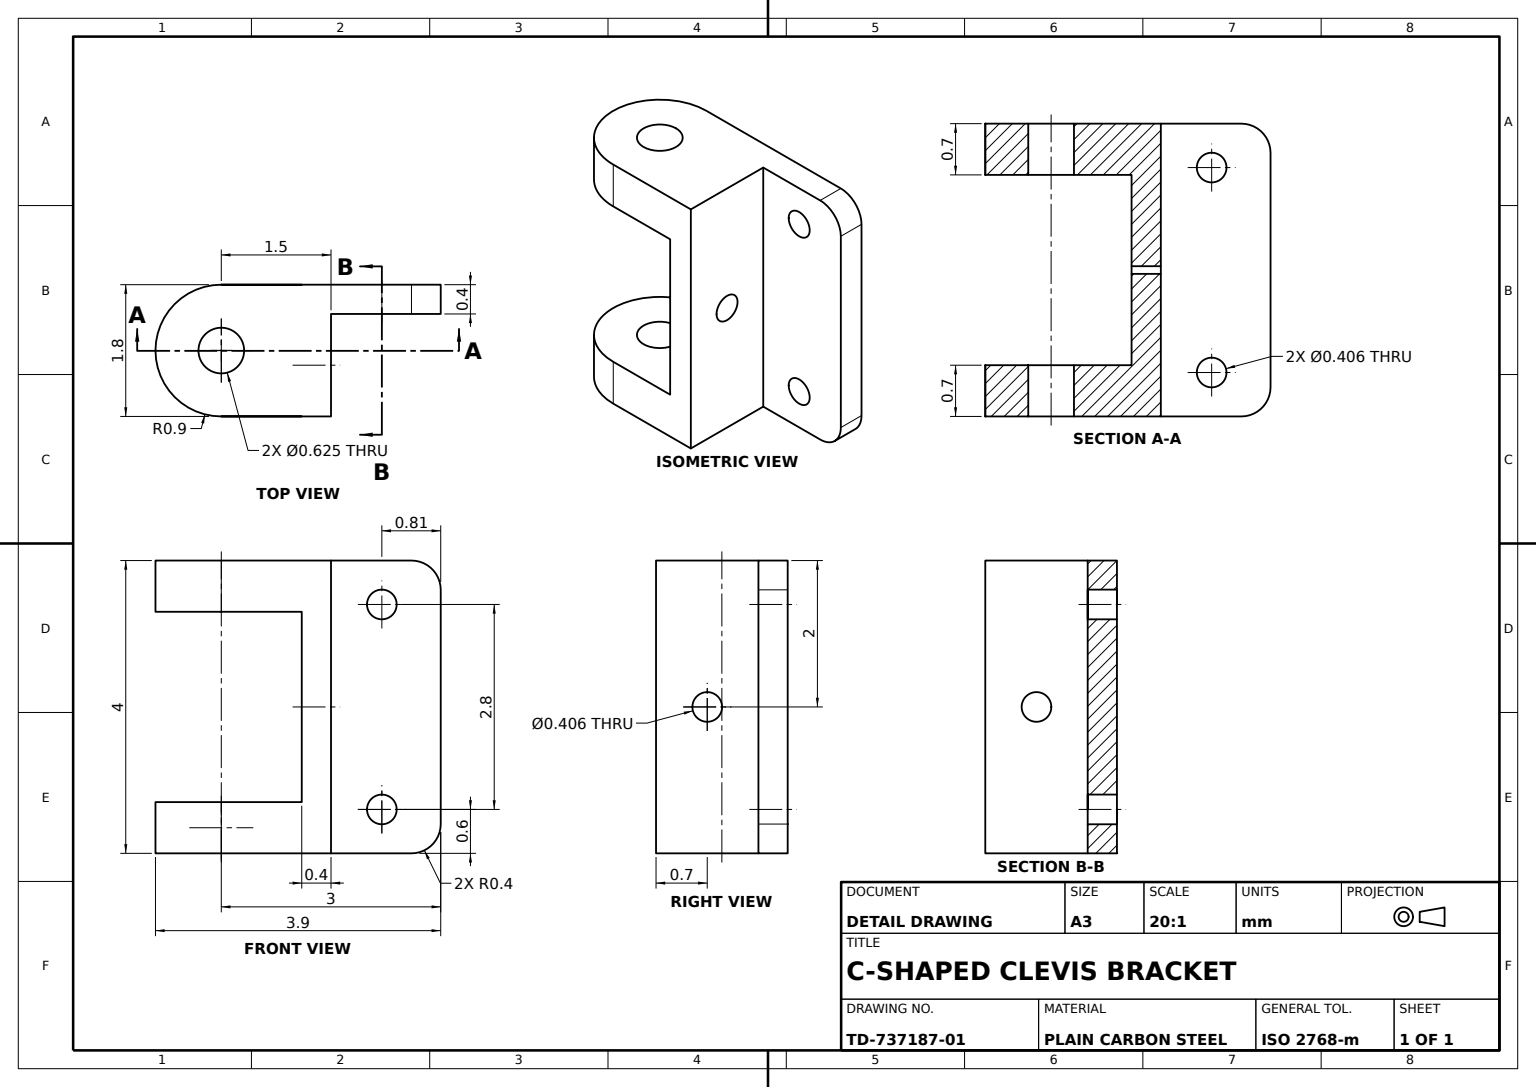
from build123d import *

# Parameters (mm, degrees)
C_FRAME_BASE_DEPTH       = 0.4
CLEVIS_GAP_SKETCH_W      = 0.4
CLEVIS_GAP_SKETCH_H      = 4
CLEVIS_GAP_CUT_DEPTH     = 1.5
CLEVIS_ARM_1_DEPTH       = 0.7
CLEVIS_START             = -0.7
CLEVIS_ARM_2_DEPTH       = 0.7
MOUNTING_FLANGE_SKETCH_W = 1.8
MOUNTING_FLANGE_SKETCH_H = 2.6
MOUNTING_FLANGE_DEPTH    = 0.4
BACK_WALL_HOLE_SKETCH_R  = 0.203
BACK_WALL_HOLE_DEPTH     = 0.4
FLANGE_HOLES_SKETCH_R    = 0.203
FLANGE_HOLES_2X_DEPTH    = 0.4
ARM_1_PIN_HOLE_SKETCH_R  = 0.3125
ARM_1_PIN_HOLE_DEPTH     = 0.7
ARM_START                = -0.7
ARM_2_PIN_HOLE_SKETCH_R  = 0.3125
ARM_2_PIN_HOLE_DEPTH     = 0.7


with BuildPart() as part:
    # C-Frame Profile Sketch → C-Frame Base (new body)
    with BuildSketch(Plane.XY):
        with BuildLine():
            ThreePointArc((3, -3.6), (2.882842712, -3.882842712), (2.6, -4))
            Line((2.6, -4), (0, -4))
            Line((0, -4), (0, 0))
            Line((0, 0), (2.6, 0))
            ThreePointArc((2.6, 0), (2.882842712, -0.117157288), (3, -0.4))
            Line((3, -0.4), (3, -3.6))
        make_face()
    extrude(amount=C_FRAME_BASE_DEPTH)

    # Clevis Gap Sketch → Clevis Gap Cut (cut)
    with BuildSketch(Plane.ZY):
        with Locations((0.2, -2)):
            Rectangle(CLEVIS_GAP_SKETCH_W, CLEVIS_GAP_SKETCH_H)
    extrude(amount=-CLEVIS_GAP_CUT_DEPTH, mode=Mode.SUBTRACT)

    # Clevis Arm 1 Sketch → Clevis Arm 1 (add)
    with BuildSketch(Plane(origin=(0, 0, 0), x_dir=(1, 0, 0), z_dir=(0, 1, 0))):
        with BuildLine():
            Line((1.5, 0), (0, 0))
            ThreePointArc((0, 0), (-0.9, -0.9), (0, -1.8))
            Line((0, -1.8), (1.5, -1.8))
            Line((1.5, -1.8), (1.5, 0))
        make_face()
    extrude(amount=-CLEVIS_ARM_1_DEPTH)

    # Clevis Arm 2 Sketch → Clevis Arm 2 (add)
    with BuildSketch(Plane.XZ.offset(4).offset(CLEVIS_START)):
        with BuildLine():
            Line((1.5, 0), (0, 0))
            ThreePointArc((0, 0), (-0.9, 0.9), (0, 1.8))
            Line((0, 1.8), (1.5, 1.8))
            Line((1.5, 1.8), (1.5, 0))
        make_face()
    extrude(amount=CLEVIS_ARM_2_DEPTH)

    # Mounting Flange Sketch → Mounting Flange (add)
    with BuildSketch(Plane.ZY.offset(-1.5)):
        with Locations((0.9, -2)):
            Rectangle(MOUNTING_FLANGE_SKETCH_W, MOUNTING_FLANGE_SKETCH_H)
    extrude(amount=MOUNTING_FLANGE_DEPTH)

    # Back Wall Hole Sketch → Back Wall Hole (cut)
    with BuildSketch(Plane(origin=(1.5, 0, 0), x_dir=(0, 0, -1), z_dir=(1, 0, 0))):
        with Locations((-1.1, -2)):
            Circle(BACK_WALL_HOLE_SKETCH_R)
    extrude(amount=-BACK_WALL_HOLE_DEPTH, mode=Mode.SUBTRACT)

    # Flange Holes Sketch → Flange Holes 2x (cut)
    with BuildSketch(Plane.XY.offset(0.4)):
        with Locations((2.195, -0.6)):
            Circle(FLANGE_HOLES_SKETCH_R)
        with Locations((2.195, -3.4)):
            Circle(FLANGE_HOLES_SKETCH_R)
    extrude(amount=-FLANGE_HOLES_2X_DEPTH, mode=Mode.SUBTRACT)

    # Arm 1 Pin Hole Sketch → Arm 1 Pin Hole (cut)
    with BuildSketch(Plane(origin=(0, 0, 0), x_dir=(1, 0, 0), z_dir=(0, 1, 0))):
        with Locations(Location((0, -0.9, 0), (0, 0, 270))):
            Circle(ARM_1_PIN_HOLE_SKETCH_R)
    extrude(amount=-ARM_1_PIN_HOLE_DEPTH, mode=Mode.SUBTRACT)

    # Arm 2 Pin Hole Sketch → Arm 2 Pin Hole (cut)
    with BuildSketch(Plane.XZ.offset(4).offset(ARM_START)):
        with Locations(Location((0, 0.9, 0), (0, 0, 90))):
            Circle(ARM_2_PIN_HOLE_SKETCH_R)
    extrude(amount=ARM_2_PIN_HOLE_DEPTH, mode=Mode.SUBTRACT)


solid = part.part
